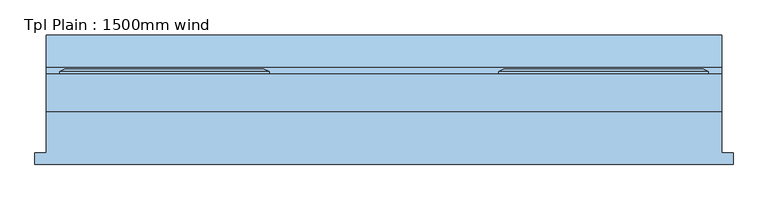
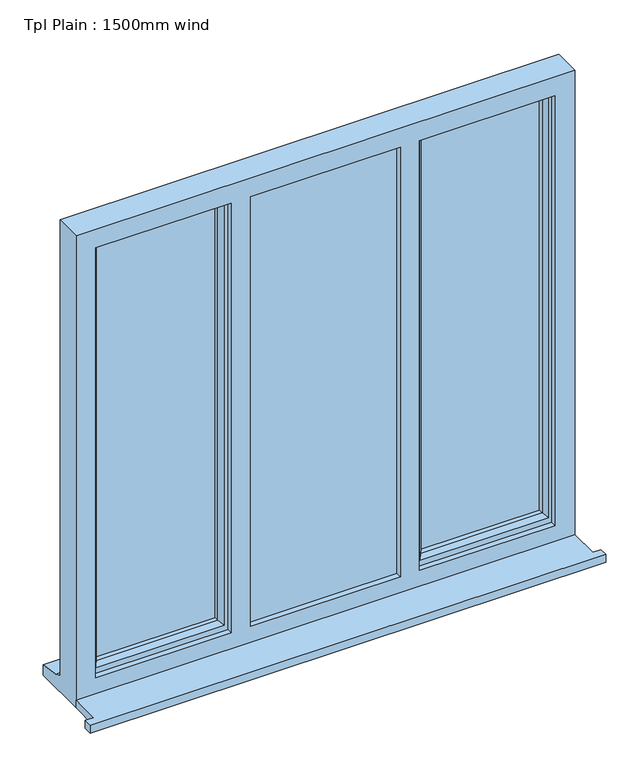
"""IFC4 building model written with IfcOpenShell, lengths in millimetres: window geometry, Tpl Plain : 1500mm wind."""

from ifc_helpers import new_model, si_unit, frame, origin, place, context, project, spatial, polyline, outline, extrude, faceted_brep, source, transform, mapped, element, save


def tpl_plain_1500mm_wind_d4a9cd4c(model_context):
    return source(origin(), model_context, "Body", "SolidModel", [
        extrude(outline(polyline([(-1300.0, -129.0434322), (-1300.0, -104.0434322), (-1275.0, -104.0434322), (-1275.0, -12.0434322), (225.0, -12.0434322), (225.0, -104.0434322), (250.0, -104.0434322), (250.0, -129.0434322), (-1300.0, -129.0434322)])), frame((0.0, 0.0, 900.0), z_axis=(0.0, 0.0, 1.0), x_axis=(1.0, 0.0, 0.0)), (0.0, 0.0, 1.0), 25.0),
        faceted_brep([(-270.0, 70.9565678, 2370.0), (-270.0, 76.7300705, 2370.0), (-270.0, 76.7300705, 953.0), (-270.0, 70.9565678, 953.0), (-260.0, 5.9565678, 2360.0), (-260.0, 70.9565678, 2360.0), (-260.0, 70.9565678, 963.0), (-260.0, 5.9565678, 963.0), (-220.0, 20.4494677, 2320.0), (-230.1480377, 5.9565678, 2330.1480377), (-230.1480377, 5.9565678, 992.8519623), (-220.0, 20.4494677, 1003.0), (-220.0, 34.9565678, 2320.0), (-220.0, 34.9565678, 1003.0), (-230.0, 58.9565678, 2330.0), (-230.0, 34.9565678, 2330.0), (-230.0, 34.9565678, 993.0), (-230.0, 58.9565678, 993.0), (-220.0, 76.7300705, 2320.0), (-220.0, 58.9565678, 2320.0), (-220.0, 58.9565678, 1003.0), (-220.0, 76.7300705, 1003.0), (-237.4457548, 82.5035732, 2337.4457548), (-237.4457548, 82.5035732, 985.5542452), (-259.2153903, 82.5035732, 2359.2153903), (-259.2153903, 82.5035732, 963.7846097), (195.0, 76.7300705, 953.0), (195.0, 70.9565678, 953.0), (185.0, 70.9565678, 963.0), (185.0, 5.9565678, 963.0), (155.1480377, 5.9565678, 992.8519623), (145.0, 20.4494677, 1003.0), (145.0, 34.9565678, 1003.0), (155.0, 34.9565678, 993.0), (155.0, 58.9565678, 993.0), (145.0, 58.9565678, 1003.0), (145.0, 76.7300705, 1003.0), (162.4457548, 82.5035732, 985.5542452), (184.2153903, 82.5035732, 963.7846097), (195.0, 76.7300705, 2370.0), (195.0, 70.9565678, 2370.0), (185.0, 70.9565678, 2360.0), (185.0, 5.9565678, 2360.0), (155.1480377, 5.9565678, 2330.1480377), (145.0, 20.4494677, 2320.0), (145.0, 34.9565678, 2320.0), (155.0, 34.9565678, 2330.0), (155.0, 58.9565678, 2330.0), (145.0, 58.9565678, 2320.0), (145.0, 76.7300705, 2320.0), (162.4457548, 82.5035732, 2337.4457548), (184.2153903, 82.5035732, 2359.2153903)], [[[0, 1, 2, 3]], [[4, 5, 6, 7]], [[8, 9, 10, 11]], [[12, 8, 11, 13]], [[14, 15, 16, 17]], [[18, 19, 20, 21]], [[22, 18, 21, 23]], [[1, 24, 25, 2]], [[3, 2, 26, 27]], [[7, 6, 28, 29]], [[11, 10, 30, 31]], [[13, 11, 31, 32]], [[17, 16, 33, 34]], [[21, 20, 35, 36]], [[23, 21, 36, 37]], [[2, 25, 38, 26]], [[27, 26, 39, 40]], [[29, 28, 41, 42]], [[31, 30, 43, 44]], [[32, 31, 44, 45]], [[34, 33, 46, 47]], [[36, 35, 48, 49]], [[37, 36, 49, 50]], [[26, 38, 51, 39]], [[40, 39, 1, 0]], [[3, 27, 40, 0], [5, 41, 28, 6]], [[42, 41, 5, 4]], [[7, 29, 42, 4], [9, 43, 30, 10]], [[44, 43, 9, 8]], [[45, 44, 8, 12]], [[15, 46, 33, 16], [13, 32, 45, 12]], [[47, 46, 15, 14]], [[17, 34, 47, 14], [19, 48, 35, 20]], [[49, 48, 19, 18]], [[50, 49, 18, 22]], [[24, 51, 38, 25], [23, 37, 50, 22]], [[39, 51, 24, 1]]]),
        faceted_brep([(-780.0, 70.9565678, 2370.0), (-780.0, 76.7300705, 2370.0), (-1245.0, 76.7300705, 2370.0), (-1245.0, 70.9565678, 2370.0), (-790.0, 5.9565678, 2360.0), (-790.0, 70.9565678, 2360.0), (-1235.0, 70.9565678, 2360.0), (-1235.0, 5.9565678, 2360.0), (-830.0, 20.4494677, 2320.0), (-819.8519623, 5.9565678, 2330.1480377), (-1205.1480377, 5.9565678, 2330.1480377), (-1195.0, 20.4494677, 2320.0), (-830.0, 34.9565678, 2320.0), (-1195.0, 34.9565678, 2320.0), (-820.0, 58.9565678, 2330.0), (-820.0, 34.9565678, 2330.0), (-1205.0, 34.9565678, 2330.0), (-1205.0, 58.9565678, 2330.0), (-830.0, 76.7300705, 2320.0), (-830.0, 58.9565678, 2320.0), (-1195.0, 58.9565678, 2320.0), (-1195.0, 76.7300705, 2320.0), (-811.1854344, 82.5035732, 2338.8145656), (-1213.8145656, 82.5035732, 2338.8145656), (-791.6307806, 82.5035732, 2358.3692194), (-1233.3692194, 82.5035732, 2358.3692194), (-1245.0, 76.7300705, 953.0), (-1245.0, 70.9565678, 953.0), (-1235.0, 70.9565678, 963.0), (-1235.0, 5.9565678, 963.0), (-1205.1480377, 5.9565678, 992.8519623), (-1195.0, 20.4494677, 1003.0), (-1195.0, 34.9565678, 1003.0), (-1205.0, 34.9565678, 993.0), (-1205.0, 58.9565678, 993.0), (-1195.0, 58.9565678, 1003.0), (-1195.0, 76.7300705, 1003.0), (-1213.8145656, 82.5035732, 984.1854344), (-1233.3692194, 82.5035732, 964.6307806), (-780.0, 76.7300705, 953.0), (-780.0, 70.9565678, 953.0), (-790.0, 70.9565678, 963.0), (-790.0, 5.9565678, 963.0), (-819.8519623, 5.9565678, 992.8519623), (-830.0, 20.4494677, 1003.0), (-830.0, 34.9565678, 1003.0), (-820.0, 34.9565678, 993.0), (-820.0, 58.9565678, 993.0), (-830.0, 58.9565678, 1003.0), (-830.0, 76.7300705, 1003.0), (-811.1854344, 82.5035732, 984.1854344), (-791.6307806, 82.5035732, 964.6307806)], [[[0, 1, 2, 3]], [[4, 5, 6, 7]], [[8, 9, 10, 11]], [[12, 8, 11, 13]], [[14, 15, 16, 17]], [[18, 19, 20, 21]], [[22, 18, 21, 23]], [[1, 24, 25, 2]], [[3, 2, 26, 27]], [[7, 6, 28, 29]], [[11, 10, 30, 31]], [[13, 11, 31, 32]], [[17, 16, 33, 34]], [[21, 20, 35, 36]], [[23, 21, 36, 37]], [[2, 25, 38, 26]], [[27, 26, 39, 40]], [[0, 3, 27, 40], [41, 28, 6, 5]], [[29, 28, 41, 42]], [[4, 7, 29, 42], [43, 30, 10, 9]], [[31, 30, 43, 44]], [[32, 31, 44, 45]], [[46, 33, 16, 15], [12, 13, 32, 45]], [[34, 33, 46, 47]], [[14, 17, 34, 47], [48, 35, 20, 19]], [[36, 35, 48, 49]], [[37, 36, 49, 50]], [[51, 38, 25, 24], [22, 23, 37, 50]], [[26, 38, 51, 39]], [[40, 39, 1, 0]], [[42, 41, 5, 4]], [[44, 43, 9, 8]], [[45, 44, 8, 12]], [[47, 46, 15, 14]], [[49, 48, 19, 18]], [[50, 49, 18, 22]], [[39, 51, 24, 1]]]),
        faceted_brep([(225.0, -12.0434322, 2400.0), (-1275.0, -12.0434322, 2400.0), (-1275.0, -12.0434322, 900.0), (225.0, -12.0434322, 900.0), (165.0, -12.0434322, 2340.0), (165.0, -12.0434322, 975.0), (-242.0, -12.0434322, 975.0), (-242.0, -12.0434322, 2340.0), (-300.0, -12.0434322, 2340.0), (-300.0, -12.0434322, 975.0), (-750.0, -12.0434322, 975.0), (-750.0, -12.0434322, 2340.0), (-808.0, -12.0434322, 2340.0), (-808.0, -12.0434322, 975.0), (-1215.0, -12.0434322, 975.0), (-1215.0, -12.0434322, 2340.0), (-1275.0, 70.9565678, 2400.0), (-1275.0, 70.9565678, 951.0), (-1275.0, 85.9565678, 949.68767), (-1275.0, 85.9565678, 944.7449676), (-1275.0, 158.4565678, 933.8088847), (-1275.0, 158.4565678, 900.0), (225.0, 70.9565678, 2400.0), (225.0, 70.9565678, 951.0), (-1235.0, 70.9565678, 2360.0), (-1235.0, 70.9565678, 963.0), (-790.0, 70.9565678, 963.0), (-790.0, 70.9565678, 2360.0), (-750.0, 70.9565678, 2360.0), (-750.0, 70.9565678, 963.0), (-300.0, 70.9565678, 963.0), (-300.0, 70.9565678, 2360.0), (-260.0, 70.9565678, 2360.0), (-260.0, 70.9565678, 963.0), (185.0, 70.9565678, 963.0), (185.0, 70.9565678, 2360.0), (-1235.0, 5.9565678, 2360.0), (-1235.0, 5.9565678, 963.0), (-760.0, 5.9565678, 2360.0), (-290.0, 5.9565678, 2360.0), (-290.0, 5.9565678, 963.0), (-760.0, 5.9565678, 963.0), (-300.0, 5.9565678, 2340.0), (-750.0, 5.9565678, 2340.0), (-750.0, 5.9565678, 975.0), (-300.0, 5.9565678, 975.0), (-260.0, 5.9565678, 2360.0), (185.0, 5.9565678, 2360.0), (185.0, 5.9565678, 963.0), (-260.0, 5.9565678, 963.0), (165.0, 5.9565678, 2340.0), (-242.0, 5.9565678, 2340.0), (-242.0, 5.9565678, 975.0), (165.0, 5.9565678, 975.0), (-790.0, 5.9565678, 2360.0), (-790.0, 5.9565678, 963.0), (-808.0, 5.9565678, 2340.0), (-1215.0, 5.9565678, 2340.0), (-1215.0, 5.9565678, 975.0), (-808.0, 5.9565678, 975.0), (-750.0, 29.9565678, 2360.0), (-300.0, 29.9565678, 2360.0), (-290.0, 29.9565678, 2360.0), (-760.0, 29.9565678, 2360.0), (225.0, 158.4565678, 900.0), (225.0, 158.4565678, 933.8088847), (225.0, 85.9565678, 944.7449676), (225.0, 85.9565678, 949.68767), (-750.0, 29.9565678, 963.0), (-760.0, 29.9565678, 963.0), (-290.0, 29.9565678, 963.0), (-300.0, 29.9565678, 963.0)], [[[0, 1, 2, 3], [4, 5, 6, 7], [8, 9, 10, 11], [12, 13, 14, 15]], [[2, 1, 16, 17, 18, 19, 20, 21]], [[17, 16, 22, 23], [24, 25, 26, 27], [28, 29, 30, 31], [32, 33, 34, 35]], [[25, 24, 36, 37]], [[38, 39, 40, 41], [42, 43, 44, 45]], [[46, 47, 48, 49], [50, 51, 52, 53]], [[36, 54, 55, 37], [56, 57, 58, 59]], [[57, 15, 14, 58]], [[1, 0, 22, 16]], [[36, 24, 27, 54]], [[35, 47, 46, 32]], [[60, 28, 31, 61, 62, 39, 38, 63]], [[15, 57, 56, 12]], [[50, 4, 7, 51]], [[11, 43, 42, 8]], [[23, 22, 0, 3, 64, 65, 66, 67]], [[35, 34, 48, 47]], [[4, 50, 53, 5]], [[43, 11, 10, 44]], [[12, 56, 59, 13]], [[27, 26, 55, 54]], [[29, 28, 60, 68]], [[68, 60, 63, 69]], [[69, 63, 38, 41]], [[62, 70, 40, 39]], [[70, 62, 61, 71]], [[71, 61, 31, 30]], [[33, 32, 46, 49]], [[51, 7, 6, 52]], [[8, 42, 45, 9]], [[64, 3, 2, 21]], [[65, 64, 21, 20]], [[66, 65, 20, 19]], [[67, 66, 19, 18]], [[23, 67, 18, 17]], [[26, 25, 37, 55]], [[34, 33, 49, 48]], [[41, 40, 70, 71, 30, 29, 68, 69]], [[6, 5, 53, 52]], [[45, 44, 10, 9]], [[59, 58, 14, 13]]]),
        extrude(outline(polyline([(-820.0, 34.9565678), (-1205.0, 34.9565678), (-1205.0, 58.9565678), (-820.0, 58.9565678), (-820.0, 34.9565678)])), frame((0.0, 0.0, 993.0), z_axis=(0.0, 0.0, 1.0), x_axis=(1.0, 0.0, 0.0)), (0.0, 0.0, 1.0), 1337.0),
        extrude(outline(polyline([(-760.0, 29.9565678), (-290.0, 29.9565678), (-290.0, 5.9565678), (-760.0, 5.9565678), (-760.0, 29.9565678)])), frame((0.0, 0.0, 963.0), z_axis=(0.0, 0.0, 1.0), x_axis=(1.0, 0.0, 0.0)), (0.0, 0.0, 1.0), 1397.0),
        extrude(outline(polyline([(155.0, 34.9565678), (-230.0, 34.9565678), (-230.0, 58.9565678), (155.0, 58.9565678), (155.0, 34.9565678)])), frame((0.0, 0.0, 993.0), z_axis=(0.0, 0.0, 1.0), x_axis=(1.0, 0.0, 0.0)), (0.0, 0.0, 1.0), 1337.0),
    ])


if __name__ == "__main__":
    model = new_model("IFC4")
    model_context = context("Model", 3, world=origin())
    ifc_project = project(units=[si_unit("LENGTHUNIT", "METRE", prefix="MILLI")], contexts=[model_context])
    site = spatial("IfcSite", under=ifc_project)
    building = spatial("IfcBuilding", under=site)
    placement = place(None, origin())
    tpl_plain_1500mm_wind_shape = tpl_plain_1500mm_wind_d4a9cd4c(model_context)
    element("IfcWindow", 1, ObjectType="Tpl Plain : 1500mm wind", at=placement, inside=building, context=model_context, shape_type="MappedRepresentation", body=[
        mapped(tpl_plain_1500mm_wind_shape, transform((0.0, 0.0, 0.0), x_axis=(1.0, 0.0, 0.0), y_axis=(0.0, 1.0, 0.0), z_axis=(0.0, 0.0, 1.0))),
    ])
    save(model, "model.ifc")

# Revit data of these elements
# Type "Tpl Plain : 1500mm wind"
#   Type Mark = "34"
#   Operation = "TriplePanelVertical"
#   Manufacturer = "Revit"
#   Keynote = "L10"
#   Analytic Construction = "<None>"
#   Wrap Layers (Ext) from Ext = 102.5 mm
#   Wrap Layers (Int) from Ext = 177.5 mm
#   Window Board Projection = 25 mm
#   Window Board Extension = 25 mm
#   Rough Width = 1500 mm
#   Rough Height = 1500 mm
#   Height = 1500 mm
#   Width = 1500 mm
#   Glazing Thickness = 24 mm
#   FrameOffset - External = 50 mm
#   Frame Depth = 65 mm
#   Default Head Height = 2400 mm
#   Cill Depth = 87.5 mm
#   Cavity Closer Width = 50 mm
#   Cavity Closer Offset from Ext = 102.5 mm
#   Cavity Closer Depth = 85 mm
#   Vis - Cavity Closers = yes
#   Define Thermal Properties by = 1
#   Material Trim = Window Frame
#   Material Glass = Glass
#   Material Frame = Window Frame
#   Wall Closure = (empty or 0)
# Element 1 (IfcWindow, "Tpl Plain : 1500mm wind")
#   Materials on its faces: "Window Frame", "Glass"
# Materials
#   "Window Frame": colour RGB 249 249 249, transparency 0, Keynote = "L10", Cost = 0
#   "Glass": class "Glass", colour RGB 0 128 192, transparency 0.9, Description = "Soda Lime Glass", Cost = 0
